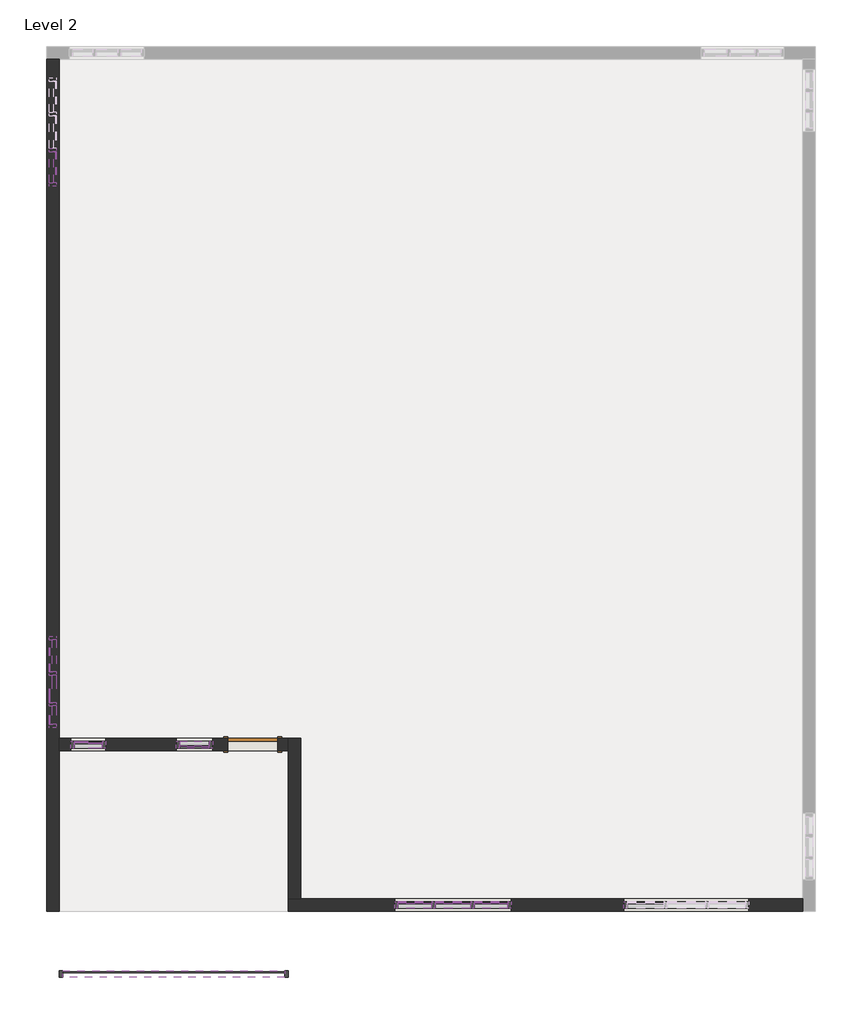
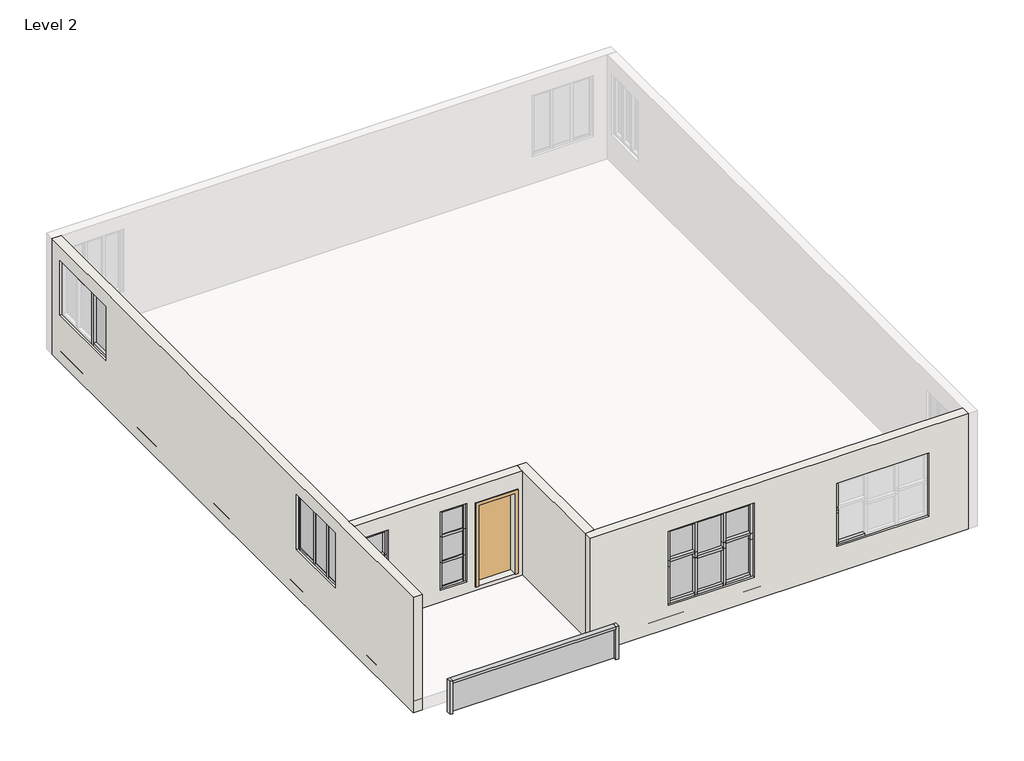
# One storey, part 1 of 2: 64 members, 17 plates, 4 walls, 1 door.
"""IFC4 building model written with IfcOpenShell, lengths in millimetres."""

from ifc_helpers import new_model, si_unit, frame, origin, place, context, project, spatial, polyline, outline, extrude, faceted_brep, transform, mapped, element, save
from components import door_0ca8825f, member_2ebf4a73, member_c33c434a, member_7fd687a9, member_90750a43, member_e53b78c9, member_5215b92c, member_3f0e0172, member_f6f0dfdd, member_f8dc38bf, member_876f8f00, member_a400357f, member_6f432376, member_04a79ac1, member_b1615173, member_02b8d6b6, member_e5d39754, member_6045db05, member_ce41b455, member_0c7d0587, member_4df5bd8f, member_19666b72, member_6e6cbf30, member_3d7cb871, member_3cc62806, member_2ad165f7, member_377cf5f8, member_b281fab0, member_bdfbb35d, member_c769c9ba, member_bec57569, member_6f9d7b88, system_panel_glazed_a7448bf8, system_panel_glazed_e40eab22, system_panel_glazed_7c0c5eec, system_panel_glazed_eaaab531, system_panel_glazed_8162a39b, system_panel_glazed_8a587fcc, system_panel_glazed_8182dcf9, system_panel_glazed_b409b60d, system_panel_glazed_f2280d1b, system_panel_glazed_618baec5, system_panel_glazed_209ba7b6, system_panel_glazed_68ae91f2, system_panel_glazed_7aae5990

model = new_model("IFC4")

# Units and contexts
model_context = context("Model", 3, world=origin())
ifc_project = project(units=[si_unit("LENGTHUNIT", "METRE", prefix="MILLI")], contexts=[model_context])

# Site, building, storey
site = spatial("IfcSite", under=ifc_project)
building = spatial("IfcBuilding", under=site)
storey = spatial("IfcBuildingStorey", under=building, Name="Level 2", Elevation=3048.0)

# Door
placement = place(None, origin())
door_shape = door_0ca8825f(model_context)
element("IfcDoor", 1, ObjectType="Single-Flush : 36\" x 84\"", at=placement, inside=storey, context=model_context, shape_type="MappedRepresentation", body=[
    mapped(door_shape, transform((-18079.9097681, -11198.7339922, 3454.4), x_axis=(1.0, 0.0, 0.0), y_axis=(0.0, 1.0, 0.0), z_axis=(0.0, 0.0, 1.0))),
])

# Members
member_shape = member_2ebf4a73(model_context)
element("IfcMember", 2, ObjectType="Rectangular Mullion : 2.5\" x 5\" rectangular", at=placement, inside=storey, context=model_context, shape_type="MappedRepresentation", body=[
    mapped(member_shape, transform((-21737.5097681, -9935.0839922, 5757.8760039), x_axis=(0.0, 0.0, 1.0), y_axis=(1.0, 0.0, 0.0), z_axis=(0.0, 1.0, 0.0))),
])
element("IfcMember", 3, ObjectType="Rectangular Mullion : 2.5\" x 5\" rectangular", at=placement, inside=storey, context=model_context, shape_type="MappedRepresentation", body=[
    mapped(member_shape, transform((-21737.5097681, -10430.3839922, 4301.2247959), x_axis=(0.0, 0.0, -1.0), y_axis=(1.0, 0.0, 0.0), z_axis=(0.0, -1.0, 0.0))),
])
member_2_shape = member_c33c434a(model_context)
element("IfcMember", 4, ObjectType="Rectangular Mullion : 2.5\" x 5\" rectangular", at=placement, inside=storey, context=model_context, shape_type="MappedRepresentation", body=[
    mapped(member_2_shape, transform((-11234.6097681, -14132.4339922, 3732.481147), x_axis=(0.0, 0.0, -1.0), y_axis=(0.0, -1.0, 0.0), z_axis=(-1.0, 0.0, 0.0))),
])
member_3_shape = member_7fd687a9(model_context)
element("IfcMember", 5, ObjectType="Rectangular Mullion : 2.5\" x 5\" rectangular", at=placement, inside=storey, context=model_context, shape_type="MappedRepresentation", body=[
    mapped(member_3_shape, transform((-20835.8097681, -11198.7339922, 5713.3390555), x_axis=(0.0, 0.0, 1.0), y_axis=(0.0, -1.0, 0.0), z_axis=(1.0, 0.0, 0.0))),
])
member_4_shape = member_90750a43(model_context)
element("IfcMember", 6, ObjectType="Rectangular Mullion : 2.5\" x 5\" rectangular", at=placement, inside=storey, context=model_context, shape_type="MappedRepresentation", body=[
    mapped(member_4_shape, transform((-20835.8097681, -11198.7339922, 5044.6242619), x_axis=(0.0, 0.0, 1.0), y_axis=(0.0, -1.0, 0.0), z_axis=(1.0, 0.0, 0.0))),
])
element("IfcMember", 7, ObjectType="Rectangular Mullion : 2.5\" x 5\" rectangular", at=placement, inside=storey, context=model_context, shape_type="MappedRepresentation", body=[
    mapped(member_4_shape, transform((-20835.8097681, -11198.7339922, 4375.9094684), x_axis=(0.0, 0.0, 1.0), y_axis=(0.0, -1.0, 0.0), z_axis=(1.0, 0.0, 0.0))),
])
element("IfcMember", 8, ObjectType="Rectangular Mullion : 2.5\" x 5\" rectangular", at=placement, inside=storey, context=model_context, shape_type="MappedRepresentation", body=[
    mapped(member_3_shape, transform((-21343.8097681, -11198.7339922, 3707.1946748), x_axis=(0.0, 0.0, -1.0), y_axis=(0.0, -1.0, 0.0), z_axis=(-1.0, 0.0, 0.0))),
])
member_5_shape = member_e53b78c9(model_context)
element("IfcMember", 9, ObjectType="Rectangular Mullion : 2.5\" x 5\" rectangular", at=placement, inside=storey, context=model_context, shape_type="MappedRepresentation", body=[
    mapped(member_5_shape, transform((-14098.4597681, -14132.4339922, 4627.6072298), x_axis=(0.0, 0.0, 1.0), y_axis=(0.0, -1.0, 0.0), z_axis=(1.0, 0.0, 0.0))),
])
member_6_shape = member_5215b92c(model_context)
element("IfcMember", 10, ObjectType="Rectangular Mullion : 2.5\" x 5\" rectangular", at=placement, inside=storey, context=model_context, shape_type="MappedRepresentation", body=[
    mapped(member_6_shape, transform((-14098.4597681, -14132.4339922, 5607.3382011), x_axis=(0.0, 0.0, 1.0), y_axis=(0.0, -1.0, 0.0), z_axis=(1.0, 0.0, 0.0))),
])
member_7_shape = member_3f0e0172(model_context)
element("IfcMember", 11, ObjectType="Rectangular Mullion : 2.5\" x 5\" rectangular", at=placement, inside=storey, context=model_context, shape_type="MappedRepresentation", body=[
    mapped(member_7_shape, transform((-14809.6597681, -14132.4339922, 5607.3382011), x_axis=(0.0, 0.0, 1.0), y_axis=(0.0, -1.0, 0.0), z_axis=(1.0, 0.0, 0.0))),
])
element("IfcMember", 12, ObjectType="Rectangular Mullion : 2.5\" x 5\" rectangular", at=placement, inside=storey, context=model_context, shape_type="MappedRepresentation", body=[
    mapped(member_7_shape, transform((-13419.0097681, -14132.4339922, 5607.3382011), x_axis=(0.0, 0.0, 1.0), y_axis=(0.0, -1.0, 0.0), z_axis=(1.0, 0.0, 0.0))),
])
member_8_shape = member_f6f0dfdd(model_context)
element("IfcMember", 13, ObjectType="Rectangular Mullion : 2.5\" x 5\" rectangular", at=placement, inside=storey, context=model_context, shape_type="MappedRepresentation", body=[
    mapped(member_8_shape, transform((-14777.9097681, -14132.4339922, 4627.6072298), x_axis=(1.0, 0.0, 0.0), y_axis=(0.0, -1.0, 0.0), z_axis=(0.0, 0.0, -1.0))),
])
element("IfcMember", 14, ObjectType="Rectangular Mullion : 2.5\" x 5\" rectangular", at=placement, inside=storey, context=model_context, shape_type="MappedRepresentation", body=[
    mapped(member_8_shape, transform((-14066.7097681, -14132.4339922, 4627.6072298), x_axis=(1.0, 0.0, 0.0), y_axis=(0.0, -1.0, 0.0), z_axis=(0.0, 0.0, -1.0))),
])
member_9_shape = member_f8dc38bf(model_context)
element("IfcMember", 15, ObjectType="Rectangular Mullion : 2.5\" x 5\" rectangular", at=placement, inside=storey, context=model_context, shape_type="MappedRepresentation", body=[
    mapped(member_9_shape, transform((-13419.0097681, -14132.4339922, 4780.0072298), x_axis=(0.0, 0.0, 1.0), y_axis=(0.0, -1.0, 0.0), z_axis=(1.0, 0.0, 0.0))),
])
element("IfcMember", 16, ObjectType="Rectangular Mullion : 2.5\" x 5\" rectangular", at=placement, inside=storey, context=model_context, shape_type="MappedRepresentation", body=[
    mapped(member_9_shape, transform((-14809.6597681, -14132.4339922, 4780.0072298), x_axis=(0.0, 0.0, 1.0), y_axis=(0.0, -1.0, 0.0), z_axis=(1.0, 0.0, 0.0))),
])
member_10_shape = member_876f8f00(model_context)
element("IfcMember", 17, ObjectType="Rectangular Mullion : 2.5\" x 5\" rectangular", at=placement, inside=storey, context=model_context, shape_type="MappedRepresentation", body=[
    mapped(member_10_shape, transform((-13355.5097681, -14132.4339922, 4627.6072298), x_axis=(1.0, 0.0, 0.0), y_axis=(0.0, -1.0, 0.0), z_axis=(0.0, 0.0, -1.0))),
])
element("IfcMember", 18, ObjectType="Rectangular Mullion : 2.5\" x 5\" rectangular", at=placement, inside=storey, context=model_context, shape_type="MappedRepresentation", body=[
    mapped(member_10_shape, transform((-15489.1097681, -14132.4339922, 4780.0072298), x_axis=(-1.0, 0.0, 0.0), y_axis=(0.0, -1.0, 0.0), z_axis=(0.0, 0.0, 1.0))),
])
element("IfcMember", 19, ObjectType="Rectangular Mullion : 2.5\" x 5\" rectangular", at=placement, inside=storey, context=model_context, shape_type="MappedRepresentation", body=[
    mapped(member_7_shape, transform((-14034.9597681, -14132.4339922, 3647.8762585), x_axis=(0.0, 0.0, -1.0), y_axis=(0.0, -1.0, 0.0), z_axis=(-1.0, 0.0, 0.0))),
])
element("IfcMember", 20, ObjectType="Rectangular Mullion : 2.5\" x 5\" rectangular", at=placement, inside=storey, context=model_context, shape_type="MappedRepresentation", body=[
    mapped(member_7_shape, transform((-15425.6097681, -14132.4339922, 3647.8762585), x_axis=(0.0, 0.0, -1.0), y_axis=(0.0, -1.0, 0.0), z_axis=(-1.0, 0.0, 0.0))),
])
element("IfcMember", 21, ObjectType="Rectangular Mullion : 2.5\" x 5\" rectangular", at=placement, inside=storey, context=model_context, shape_type="MappedRepresentation", body=[
    mapped(member_6_shape, transform((-14746.1597681, -14132.4339922, 3647.8762585), x_axis=(0.0, 0.0, -1.0), y_axis=(0.0, -1.0, 0.0), z_axis=(-1.0, 0.0, 0.0))),
])
member_11_shape = member_a400357f(model_context)
element("IfcMember", 22, ObjectType="Rectangular Mullion : 2.5\" x 5\" rectangular", at=placement, inside=storey, context=model_context, shape_type="MappedRepresentation", body=[
    mapped(member_11_shape, transform((-21737.5097681, -295.7839922, 5718.9037492), x_axis=(0.0, 0.0, 1.0), y_axis=(-1.0, 0.0, 0.0), z_axis=(0.0, -1.0, 0.0))),
])
member_12_shape = member_6f432376(model_context)
element("IfcMember", 23, ObjectType="Rectangular Mullion : 2.5\" x 5\" rectangular", at=placement, inside=storey, context=model_context, shape_type="MappedRepresentation", body=[
    mapped(member_12_shape, transform((-21737.5097681, -924.4339922, 5718.9037492), x_axis=(0.0, 0.0, 1.0), y_axis=(-1.0, 0.0, 0.0), z_axis=(0.0, -1.0, 0.0))),
])
member_13_shape = member_04a79ac1(model_context)
element("IfcMember", 24, ObjectType="Rectangular Mullion : 2.5\" x 5\" rectangular", at=placement, inside=storey, context=model_context, shape_type="MappedRepresentation", body=[
    mapped(member_13_shape, transform((-21737.5097681, -327.5339922, 4287.8866443), x_axis=(0.0, -1.0, 0.0), y_axis=(-1.0, 0.0, 0.0), z_axis=(0.0, 0.0, -1.0))),
])
element("IfcMember", 25, ObjectType="Rectangular Mullion : 2.5\" x 5\" rectangular", at=placement, inside=storey, context=model_context, shape_type="MappedRepresentation", body=[
    mapped(member_12_shape, transform((-21737.5097681, -359.2839922, 4287.8866443), x_axis=(0.0, 0.0, -1.0), y_axis=(-1.0, 0.0, 0.0), z_axis=(0.0, 1.0, 0.0))),
])
member_14_shape = member_b1615173(model_context)
element("IfcMember", 26, ObjectType="Rectangular Mullion : 2.5\" x 5\" rectangular", at=placement, inside=storey, context=model_context, shape_type="MappedRepresentation", body=[
    mapped(member_14_shape, transform((-21737.5097681, -987.9339922, 4287.8866443), x_axis=(0.0, -1.0, 0.0), y_axis=(-1.0, 0.0, 0.0), z_axis=(0.0, 0.0, -1.0))),
])
member_15_shape = member_02b8d6b6(model_context)
element("IfcMember", 27, ObjectType="Rectangular Mullion : 2.5\" x 5\" rectangular", at=placement, inside=storey, context=model_context, shape_type="MappedRepresentation", body=[
    mapped(member_15_shape, transform((-21737.5097681, -10493.8839922, 5757.8760039), x_axis=(0.0, 0.0, 1.0), y_axis=(1.0, 0.0, 0.0), z_axis=(0.0, 1.0, 0.0))),
])
member_16_shape = member_e5d39754(model_context)
element("IfcMember", 28, ObjectType="Rectangular Mullion : 2.5\" x 5\" rectangular", at=placement, inside=storey, context=model_context, shape_type="MappedRepresentation", body=[
    mapped(member_16_shape, transform((-21737.5097681, -9281.0339922, 5757.8760039), x_axis=(0.0, 0.0, 1.0), y_axis=(1.0, 0.0, 0.0), z_axis=(0.0, 1.0, 0.0))),
])
member_17_shape = member_6045db05(model_context)
element("IfcMember", 29, ObjectType="Rectangular Mullion : 2.5\" x 5\" rectangular", at=placement, inside=storey, context=model_context, shape_type="MappedRepresentation", body=[
    mapped(member_17_shape, transform((-21737.5097681, -9903.3339922, 4301.2247959), x_axis=(0.0, 1.0, 0.0), y_axis=(1.0, 0.0, 0.0), z_axis=(0.0, 0.0, -1.0))),
])
element("IfcMember", 30, ObjectType="Rectangular Mullion : 2.5\" x 5\" rectangular", at=placement, inside=storey, context=model_context, shape_type="MappedRepresentation", body=[
    mapped(member_17_shape, transform((-21737.5097681, -10462.1339922, 4301.2247959), x_axis=(0.0, 1.0, 0.0), y_axis=(1.0, 0.0, 0.0), z_axis=(0.0, 0.0, -1.0))),
])
element("IfcMember", 31, ObjectType="Rectangular Mullion : 2.5\" x 5\" rectangular", at=placement, inside=storey, context=model_context, shape_type="MappedRepresentation", body=[
    mapped(member_16_shape, transform((-21737.5097681, -9871.5839922, 4301.2247959), x_axis=(0.0, 0.0, -1.0), y_axis=(1.0, 0.0, 0.0), z_axis=(0.0, -1.0, 0.0))),
])
element("IfcMember", 32, ObjectType="Rectangular Mullion : 2.5\" x 5\" rectangular", at=placement, inside=storey, context=model_context, shape_type="MappedRepresentation", body=[
    mapped(member_15_shape, transform((-21737.5097681, -10830.4339922, 4301.2247959), x_axis=(0.0, 0.0, -1.0), y_axis=(1.0, 0.0, 0.0), z_axis=(0.0, -1.0, 0.0))),
])
member_18_shape = member_ce41b455(model_context)
element("IfcMember", 33, ObjectType="Rectangular Mullion : 2.5\" x 5\" rectangular", at=placement, inside=storey, context=model_context, shape_type="MappedRepresentation", body=[
    mapped(member_18_shape, transform((-21737.5097681, -10893.9339922, 5757.8760039), x_axis=(0.0, -1.0, 0.0), y_axis=(1.0, 0.0, 0.0), z_axis=(0.0, 0.0, 1.0))),
])
element("IfcMember", 34, ObjectType="Rectangular Mullion : 2.5\" x 5\" rectangular", at=placement, inside=storey, context=model_context, shape_type="MappedRepresentation", body=[
    mapped(member_18_shape, transform((-21737.5097681, -9217.5339922, 4301.2247959), x_axis=(0.0, 1.0, 0.0), y_axis=(1.0, 0.0, 0.0), z_axis=(0.0, 0.0, -1.0))),
])
member_19_shape = member_0c7d0587(model_context)
element("IfcMember", 35, ObjectType="Rectangular Mullion : 2.5\" x 5\" rectangular", at=placement, inside=storey, context=model_context, shape_type="MappedRepresentation", body=[
    mapped(member_19_shape, transform((-14777.9097681, -14132.4339922, 4780.0072298), x_axis=(1.0, 0.0, 0.0), y_axis=(0.0, -1.0, 0.0), z_axis=(0.0, 0.0, -1.0))),
])
element("IfcMember", 36, ObjectType="Rectangular Mullion : 2.5\" x 5\" rectangular", at=placement, inside=storey, context=model_context, shape_type="MappedRepresentation", body=[
    mapped(member_19_shape, transform((-14066.7097681, -14132.4339922, 4780.0072298), x_axis=(1.0, 0.0, 0.0), y_axis=(0.0, -1.0, 0.0), z_axis=(0.0, 0.0, -1.0))),
])
member_20_shape = member_4df5bd8f(model_context)
element("IfcMember", 37, ObjectType="Rectangular Mullion : 2.5\" x 5\" rectangular", at=placement, inside=storey, context=model_context, shape_type="MappedRepresentation", body=[
    mapped(member_20_shape, transform((-15489.1097681, -14132.4339922, 5607.3382011), x_axis=(-1.0, 0.0, 0.0), y_axis=(0.0, -1.0, 0.0), z_axis=(0.0, 0.0, 1.0))),
])
element("IfcMember", 38, ObjectType="Rectangular Mullion : 2.5\" x 5\" rectangular", at=placement, inside=storey, context=model_context, shape_type="MappedRepresentation", body=[
    mapped(member_20_shape, transform((-13355.5097681, -14132.4339922, 4780.0072298), x_axis=(1.0, 0.0, 0.0), y_axis=(0.0, -1.0, 0.0), z_axis=(0.0, 0.0, -1.0))),
])
member_21_shape = member_19666b72(model_context)
element("IfcMember", 39, ObjectType="Rectangular Mullion : 2.5\" x 5\" rectangular", at=placement, inside=storey, context=model_context, shape_type="MappedRepresentation", body=[
    mapped(member_21_shape, transform((-14777.9097681, -14132.4339922, 3647.8762585), x_axis=(1.0, 0.0, 0.0), y_axis=(0.0, -1.0, 0.0), z_axis=(0.0, 0.0, -1.0))),
])
element("IfcMember", 40, ObjectType="Rectangular Mullion : 2.5\" x 5\" rectangular", at=placement, inside=storey, context=model_context, shape_type="MappedRepresentation", body=[
    mapped(member_21_shape, transform((-14066.7097681, -14132.4339922, 3647.8762585), x_axis=(1.0, 0.0, 0.0), y_axis=(0.0, -1.0, 0.0), z_axis=(0.0, 0.0, -1.0))),
])
member_22_shape = member_6e6cbf30(model_context)
element("IfcMember", 41, ObjectType="Rectangular Mullion : 2.5\" x 5\" rectangular", at=placement, inside=storey, context=model_context, shape_type="MappedRepresentation", body=[
    mapped(member_22_shape, transform((-15489.1097681, -14132.4339922, 4627.6072298), x_axis=(-1.0, 0.0, 0.0), y_axis=(0.0, -1.0, 0.0), z_axis=(0.0, 0.0, 1.0))),
])
element("IfcMember", 42, ObjectType="Rectangular Mullion : 2.5\" x 5\" rectangular", at=placement, inside=storey, context=model_context, shape_type="MappedRepresentation", body=[
    mapped(member_22_shape, transform((-13355.5097681, -14132.4339922, 3647.8762585), x_axis=(1.0, 0.0, 0.0), y_axis=(0.0, -1.0, 0.0), z_axis=(0.0, 0.0, -1.0))),
])
member_23_shape = member_3d7cb871(model_context)
element("IfcMember", 43, ObjectType="Rectangular Mullion : 2.5\" x 5\" rectangular", at=placement, inside=storey, context=model_context, shape_type="MappedRepresentation", body=[
    mapped(member_23_shape, transform((-11298.1097681, -14132.4339922, 4641.1200239), x_axis=(-1.0, 0.0, 0.0), y_axis=(0.0, -1.0, 0.0), z_axis=(0.0, 0.0, 1.0))),
])
element("IfcMember", 44, ObjectType="Rectangular Mullion : 2.5\" x 5\" rectangular", at=placement, inside=storey, context=model_context, shape_type="MappedRepresentation", body=[
    mapped(member_23_shape, transform((-11298.1097681, -14132.4339922, 4717.3200239), x_axis=(-1.0, 0.0, 0.0), y_axis=(0.0, -1.0, 0.0), z_axis=(0.0, 0.0, 1.0))),
])
member_24_shape = member_3cc62806(model_context)
element("IfcMember", 45, ObjectType="Rectangular Mullion : 2.5\" x 5\" rectangular", at=placement, inside=storey, context=model_context, shape_type="MappedRepresentation", body=[
    mapped(member_24_shape, transform((-11298.1097681, -14132.4339922, 5397.3589008), x_axis=(-1.0, 0.0, 0.0), y_axis=(0.0, -1.0, 0.0), z_axis=(0.0, 0.0, 1.0))),
])
member_25_shape = member_2ad165f7(model_context)
element("IfcMember", 46, ObjectType="Rectangular Mullion : 2.5\" x 5\" rectangular", at=placement, inside=storey, context=model_context, shape_type="MappedRepresentation", body=[
    mapped(member_25_shape, transform((-11298.1097681, -14132.4339922, 4564.9200239), x_axis=(-1.0, 0.0, 0.0), y_axis=(0.0, -1.0, 0.0), z_axis=(0.0, 0.0, 1.0))),
])
member_26_shape = member_377cf5f8(model_context)
element("IfcMember", 47, ObjectType="Rectangular Mullion : 2.5\" x 5\" rectangular", at=placement, inside=storey, context=model_context, shape_type="MappedRepresentation", body=[
    mapped(member_26_shape, transform((-20772.3097681, -11198.7339922, 5044.6242619), x_axis=(1.0, 0.0, 0.0), y_axis=(0.0, -1.0, 0.0), z_axis=(0.0, 0.0, -1.0))),
])
element("IfcMember", 48, ObjectType="Rectangular Mullion : 2.5\" x 5\" rectangular", at=placement, inside=storey, context=model_context, shape_type="MappedRepresentation", body=[
    mapped(member_26_shape, transform((-21407.3097681, -11198.7339922, 5713.3390555), x_axis=(-1.0, 0.0, 0.0), y_axis=(0.0, -1.0, 0.0), z_axis=(0.0, 0.0, 1.0))),
])
element("IfcMember", 49, ObjectType="Rectangular Mullion : 2.5\" x 5\" rectangular", at=placement, inside=storey, context=model_context, shape_type="MappedRepresentation", body=[
    mapped(member_26_shape, transform((-20772.3097681, -11198.7339922, 4375.9094684), x_axis=(1.0, 0.0, 0.0), y_axis=(0.0, -1.0, 0.0), z_axis=(0.0, 0.0, -1.0))),
])
element("IfcMember", 50, ObjectType="Rectangular Mullion : 2.5\" x 5\" rectangular", at=placement, inside=storey, context=model_context, shape_type="MappedRepresentation", body=[
    mapped(member_26_shape, transform((-21407.3097681, -11198.7339922, 5044.6242619), x_axis=(-1.0, 0.0, 0.0), y_axis=(0.0, -1.0, 0.0), z_axis=(0.0, 0.0, 1.0))),
])
element("IfcMember", 51, ObjectType="Rectangular Mullion : 2.5\" x 5\" rectangular", at=placement, inside=storey, context=model_context, shape_type="MappedRepresentation", body=[
    mapped(member_26_shape, transform((-20772.3097681, -11198.7339922, 3707.1946748), x_axis=(1.0, 0.0, 0.0), y_axis=(0.0, -1.0, 0.0), z_axis=(0.0, 0.0, -1.0))),
])
element("IfcMember", 52, ObjectType="Rectangular Mullion : 2.5\" x 5\" rectangular", at=placement, inside=storey, context=model_context, shape_type="MappedRepresentation", body=[
    mapped(member_26_shape, transform((-21407.3097681, -11198.7339922, 4375.9094684), x_axis=(-1.0, 0.0, 0.0), y_axis=(0.0, -1.0, 0.0), z_axis=(0.0, 0.0, 1.0))),
])
member_27_shape = member_b281fab0(model_context)
element("IfcMember", 53, ObjectType="Rectangular Mullion : 2.5\" x 5\" rectangular", at=placement, inside=storey, context=model_context, shape_type="MappedRepresentation", body=[
    mapped(member_27_shape, transform((-19413.4097681, -11198.7339922, 5730.4529017), x_axis=(0.0, 0.0, 1.0), y_axis=(0.0, 1.0, 0.0), z_axis=(-1.0, 0.0, 0.0))),
])
member_28_shape = member_bdfbb35d(model_context)
element("IfcMember", 54, ObjectType="Rectangular Mullion : 2.5\" x 5\" rectangular", at=placement, inside=storey, context=model_context, shape_type="MappedRepresentation", body=[
    mapped(member_28_shape, transform((-19413.4097681, -11198.7339922, 5039.9788679), x_axis=(0.0, 0.0, 1.0), y_axis=(0.0, 1.0, 0.0), z_axis=(-1.0, 0.0, 0.0))),
])
element("IfcMember", 55, ObjectType="Rectangular Mullion : 2.5\" x 5\" rectangular", at=placement, inside=storey, context=model_context, shape_type="MappedRepresentation", body=[
    mapped(member_28_shape, transform((-19413.4097681, -11198.7339922, 4349.5048342), x_axis=(0.0, 0.0, 1.0), y_axis=(0.0, 1.0, 0.0), z_axis=(-1.0, 0.0, 0.0))),
])
member_29_shape = member_c769c9ba(model_context)
element("IfcMember", 56, ObjectType="Rectangular Mullion : 2.5\" x 5\" rectangular", at=placement, inside=storey, context=model_context, shape_type="MappedRepresentation", body=[
    mapped(member_29_shape, transform((-18816.5097681, -11198.7339922, 5730.4529017), x_axis=(1.0, 0.0, 0.0), y_axis=(0.0, 1.0, 0.0), z_axis=(0.0, 0.0, 1.0))),
])
element("IfcMember", 57, ObjectType="Rectangular Mullion : 2.5\" x 5\" rectangular", at=placement, inside=storey, context=model_context, shape_type="MappedRepresentation", body=[
    mapped(member_29_shape, transform((-19476.9097681, -11198.7339922, 5039.9788679), x_axis=(-1.0, 0.0, 0.0), y_axis=(0.0, 1.0, 0.0), z_axis=(0.0, 0.0, -1.0))),
])
element("IfcMember", 58, ObjectType="Rectangular Mullion : 2.5\" x 5\" rectangular", at=placement, inside=storey, context=model_context, shape_type="MappedRepresentation", body=[
    mapped(member_29_shape, transform((-18816.5097681, -11198.7339922, 5039.9788679), x_axis=(1.0, 0.0, 0.0), y_axis=(0.0, 1.0, 0.0), z_axis=(0.0, 0.0, 1.0))),
])
element("IfcMember", 59, ObjectType="Rectangular Mullion : 2.5\" x 5\" rectangular", at=placement, inside=storey, context=model_context, shape_type="MappedRepresentation", body=[
    mapped(member_29_shape, transform((-19476.9097681, -11198.7339922, 4349.5048342), x_axis=(-1.0, 0.0, 0.0), y_axis=(0.0, 1.0, 0.0), z_axis=(0.0, 0.0, -1.0))),
])
element("IfcMember", 60, ObjectType="Rectangular Mullion : 2.5\" x 5\" rectangular", at=placement, inside=storey, context=model_context, shape_type="MappedRepresentation", body=[
    mapped(member_27_shape, transform((-18880.0097681, -11198.7339922, 3659.0308004), x_axis=(0.0, 0.0, -1.0), y_axis=(0.0, 1.0, 0.0), z_axis=(1.0, 0.0, 0.0))),
])
element("IfcMember", 61, ObjectType="Rectangular Mullion : 2.5\" x 5\" rectangular", at=placement, inside=storey, context=model_context, shape_type="MappedRepresentation", body=[
    mapped(member_29_shape, transform((-18816.5097681, -11198.7339922, 4349.5048342), x_axis=(1.0, 0.0, 0.0), y_axis=(0.0, 1.0, 0.0), z_axis=(0.0, 0.0, 1.0))),
])
element("IfcMember", 62, ObjectType="Rectangular Mullion : 2.5\" x 5\" rectangular", at=placement, inside=storey, context=model_context, shape_type="MappedRepresentation", body=[
    mapped(member_29_shape, transform((-19476.9097681, -11198.7339922, 3659.0308004), x_axis=(-1.0, 0.0, 0.0), y_axis=(0.0, 1.0, 0.0), z_axis=(0.0, 0.0, -1.0))),
])
member_30_shape = member_bec57569(model_context)
element("IfcMember", 63, ObjectType="Rectangular Mullion : 2.5\" x 5\" rectangular", at=placement, inside=storey, context=model_context, shape_type="MappedRepresentation", body=[
    mapped(member_30_shape, transform((-17432.2097681, -15394.0454888, 3659.0308004), x_axis=(1.0, 0.0, 0.0), y_axis=(0.0, -1.0, 0.0), z_axis=(0.0, 0.0, -1.0))),
])
member_31_shape = member_6f9d7b88(model_context)
element("IfcMember", 64, ObjectType="Rectangular Mullion : 2.5\" x 5\" rectangular", at=placement, inside=storey, context=model_context, shape_type="MappedRepresentation", body=[
    mapped(member_31_shape, transform((-17495.7097681, -15394.0454888, 4526.6965957), x_axis=(0.0, 0.0, 1.0), y_axis=(0.0, -1.0, 0.0), z_axis=(1.0, 0.0, 0.0))),
])
element("IfcMember", 65, ObjectType="Rectangular Mullion : 2.5\" x 5\" rectangular", at=placement, inside=storey, context=model_context, shape_type="MappedRepresentation", body=[
    mapped(member_30_shape, transform((-21623.2097681, -15394.0454888, 4526.6965957), x_axis=(-1.0, 0.0, 0.0), y_axis=(0.0, -1.0, 0.0), z_axis=(0.0, 0.0, 1.0))),
])

# Plates
system_panel_glazed_shape = system_panel_glazed_a7448bf8(model_context)
element("IfcPlate", 66, ObjectType="System Panel : Glazed", at=placement, inside=storey, context=model_context, shape_type="MappedRepresentation", body=[
    mapped(system_panel_glazed_shape, transform((-21737.5097681, -641.8589922, 4351.3866443), x_axis=(0.0, -1.0, 0.0), y_axis=(1.0, 0.0, 0.0), z_axis=(0.0, 0.0, 1.0))),
])
system_panel_glazed_2_shape = system_panel_glazed_e40eab22(model_context)
element("IfcPlate", 67, ObjectType="System Panel : Glazed", at=placement, inside=storey, context=model_context, shape_type="MappedRepresentation", body=[
    mapped(system_panel_glazed_2_shape, transform((-21737.5097681, -10662.1589922, 4364.7247959), x_axis=(0.0, 1.0, 0.0), y_axis=(-1.0, 0.0, 0.0), z_axis=(0.0, 0.0, 1.0))),
])
system_panel_glazed_3_shape = system_panel_glazed_7c0c5eec(model_context)
element("IfcPlate", 68, ObjectType="System Panel : Glazed", at=placement, inside=storey, context=model_context, shape_type="MappedRepresentation", body=[
    mapped(system_panel_glazed_3_shape, transform((-21737.5097681, -9576.3089922, 4364.7247959), x_axis=(0.0, 1.0, 0.0), y_axis=(-1.0, 0.0, 0.0), z_axis=(0.0, 0.0, 1.0))),
])
system_panel_glazed_4_shape = system_panel_glazed_eaaab531(model_context)
element("IfcPlate", 69, ObjectType="System Panel : Glazed", at=placement, inside=storey, context=model_context, shape_type="MappedRepresentation", body=[
    mapped(system_panel_glazed_4_shape, transform((-21737.5097681, -10182.7339922, 4364.7247959), x_axis=(0.0, 1.0, 0.0), y_axis=(-1.0, 0.0, 0.0), z_axis=(0.0, 0.0, 1.0))),
])
system_panel_glazed_5_shape = system_panel_glazed_8162a39b(model_context)
element("IfcPlate", 70, ObjectType="System Panel : Glazed", at=placement, inside=storey, context=model_context, shape_type="MappedRepresentation", body=[
    mapped(system_panel_glazed_5_shape, transform((-14422.3097681, -14132.4339922, 4659.3572298), x_axis=(1.0, 0.0, 0.0), y_axis=(0.0, 1.0, 0.0), z_axis=(0.0, 0.0, 1.0))),
])
system_panel_glazed_6_shape = system_panel_glazed_8a587fcc(model_context)
element("IfcPlate", 71, ObjectType="System Panel : Glazed", at=placement, inside=storey, context=model_context, shape_type="MappedRepresentation", body=[
    mapped(system_panel_glazed_6_shape, transform((-15117.6347681, -14132.4339922, 4811.7572298), x_axis=(1.0, 0.0, 0.0), y_axis=(0.0, 1.0, 0.0), z_axis=(0.0, 0.0, 1.0))),
])
element("IfcPlate", 72, ObjectType="System Panel : Glazed", at=placement, inside=storey, context=model_context, shape_type="MappedRepresentation", body=[
    mapped(system_panel_glazed_6_shape, transform((-13726.9847681, -14132.4339922, 4811.7572298), x_axis=(1.0, 0.0, 0.0), y_axis=(0.0, 1.0, 0.0), z_axis=(0.0, 0.0, 1.0))),
])
system_panel_glazed_7_shape = system_panel_glazed_8182dcf9(model_context)
element("IfcPlate", 73, ObjectType="System Panel : Glazed", at=placement, inside=storey, context=model_context, shape_type="MappedRepresentation", body=[
    mapped(system_panel_glazed_7_shape, transform((-15117.6347681, -14132.4339922, 3711.3762585), x_axis=(1.0, 0.0, 0.0), y_axis=(0.0, 1.0, 0.0), z_axis=(0.0, 0.0, 1.0))),
])
element("IfcPlate", 74, ObjectType="System Panel : Glazed", at=placement, inside=storey, context=model_context, shape_type="MappedRepresentation", body=[
    mapped(system_panel_glazed_7_shape, transform((-13726.9847681, -14132.4339922, 3711.3762585), x_axis=(1.0, 0.0, 0.0), y_axis=(0.0, 1.0, 0.0), z_axis=(0.0, 0.0, 1.0))),
])
system_panel_glazed_8_shape = system_panel_glazed_b409b60d(model_context)
element("IfcPlate", 75, ObjectType="System Panel : Glazed", at=placement, inside=storey, context=model_context, shape_type="MappedRepresentation", body=[
    mapped(system_panel_glazed_8_shape, transform((-14422.3097681, -14132.4339922, 3711.3762585), x_axis=(1.0, 0.0, 0.0), y_axis=(0.0, 1.0, 0.0), z_axis=(0.0, 0.0, 1.0))),
])
system_panel_glazed_9_shape = system_panel_glazed_f2280d1b(model_context)
element("IfcPlate", 76, ObjectType="System Panel : Glazed", at=placement, inside=storey, context=model_context, shape_type="MappedRepresentation", body=[
    mapped(system_panel_glazed_9_shape, transform((-21089.8097681, -11198.7339922, 3770.6946748), x_axis=(1.0, 0.0, 0.0), y_axis=(0.0, 1.0, 0.0), z_axis=(0.0, 0.0, 1.0))),
])
element("IfcPlate", 77, ObjectType="System Panel : Glazed", at=placement, inside=storey, context=model_context, shape_type="MappedRepresentation", body=[
    mapped(system_panel_glazed_9_shape, transform((-21089.8097681, -11198.7339922, 5076.3742619), x_axis=(1.0, 0.0, 0.0), y_axis=(0.0, 1.0, 0.0), z_axis=(0.0, 0.0, 1.0))),
])
system_panel_glazed_10_shape = system_panel_glazed_618baec5(model_context)
element("IfcPlate", 78, ObjectType="System Panel : Glazed", at=placement, inside=storey, context=model_context, shape_type="MappedRepresentation", body=[
    mapped(system_panel_glazed_10_shape, transform((-21089.8097681, -11198.7339922, 4407.6594684), x_axis=(1.0, 0.0, 0.0), y_axis=(0.0, 1.0, 0.0), z_axis=(0.0, 0.0, 1.0))),
])
system_panel_glazed_11_shape = system_panel_glazed_209ba7b6(model_context)
element("IfcPlate", 79, ObjectType="System Panel : Glazed", at=placement, inside=storey, context=model_context, shape_type="MappedRepresentation", body=[
    mapped(system_panel_glazed_11_shape, transform((-19146.7097681, -11198.7339922, 3722.5308004), x_axis=(-1.0, 0.0, 0.0), y_axis=(0.0, -1.0, 0.0), z_axis=(0.0, 0.0, 1.0))),
])
element("IfcPlate", 80, ObjectType="System Panel : Glazed", at=placement, inside=storey, context=model_context, shape_type="MappedRepresentation", body=[
    mapped(system_panel_glazed_11_shape, transform((-19146.7097681, -11198.7339922, 5071.7288679), x_axis=(-1.0, 0.0, 0.0), y_axis=(0.0, -1.0, 0.0), z_axis=(0.0, 0.0, 1.0))),
])
system_panel_glazed_12_shape = system_panel_glazed_68ae91f2(model_context)
element("IfcPlate", 81, ObjectType="System Panel : Glazed", at=placement, inside=storey, context=model_context, shape_type="MappedRepresentation", body=[
    mapped(system_panel_glazed_12_shape, transform((-19146.7097681, -11198.7339922, 4381.2548342), x_axis=(-1.0, 0.0, 0.0), y_axis=(0.0, -1.0, 0.0), z_axis=(0.0, 0.0, 1.0))),
])
system_panel_glazed_13_shape = system_panel_glazed_7aae5990(model_context)
element("IfcPlate", 82, ObjectType="System Panel : Glazed", at=placement, inside=storey, context=model_context, shape_type="MappedRepresentation", body=[
    mapped(system_panel_glazed_13_shape, transform((-19527.7097681, -15394.0454888, 3659.0308004), x_axis=(1.0, 0.0, 0.0), y_axis=(0.0, 1.0, 0.0), z_axis=(0.0, 0.0, 1.0))),
])

# Walls
element("IfcWall", 83, ObjectType="9\"", at=placement, inside=storey, context=model_context, shape_type="Brep", body=[
    faceted_brep([(-8021.5097681, -14018.1339922, 3048.0), (-17203.6097681, -14018.1339922, 3048.0), (-17432.2097681, -14018.1339922, 3048.0), (-17432.2097681, -14018.1339922, 6096.0), (-17203.6097681, -14018.1339922, 6096.0), (-8021.5097681, -14018.1339922, 6096.0), (-15489.1097681, -14018.1339922, 5607.3382011), (-15489.1097681, -14018.1339922, 3647.8762585), (-13355.5097681, -14018.1339922, 3647.8762585), (-13355.5097681, -14018.1339922, 5607.3382011), (-11298.1097681, -14018.1339922, 5397.3589008), (-11298.1097681, -14018.1339922, 3732.481147), (-9012.1097681, -14018.1339922, 3732.481147), (-9012.1097681, -14018.1339922, 5397.3589008), (-17432.2097681, -14246.7339922, 3048.0), (-8021.5097681, -14246.7339922, 3048.0), (-8021.5097681, -14246.7339922, 6096.0), (-17432.2097681, -14246.7339922, 6096.0), (-15489.1097681, -14246.7339922, 3647.8762585), (-15489.1097681, -14246.7339922, 5607.3382011), (-13355.5097681, -14246.7339922, 5607.3382011), (-13355.5097681, -14246.7339922, 3647.8762585), (-11298.1097681, -14246.7339922, 3732.481147), (-11298.1097681, -14246.7339922, 5397.3589008), (-9012.1097681, -14246.7339922, 5397.3589008), (-9012.1097681, -14246.7339922, 3732.481147)], [[[0, 1, 2, 3, 4, 5], [6, 7, 8, 9], [10, 11, 12, 13]], [[14, 15, 16, 17], [18, 19, 20, 21], [22, 23, 24, 25]], [[2, 1, 0, 15, 14]], [[5, 4, 3, 17, 16]], [[0, 5, 16, 15]], [[3, 2, 14, 17]], [[6, 19, 18, 7]], [[19, 6, 9, 20]], [[20, 9, 8, 21]], [[7, 18, 21, 8]], [[22, 11, 10, 23]], [[23, 10, 13, 24]], [[24, 13, 12, 25]], [[11, 22, 25, 12]]]),
])
element("IfcWall", 84, ObjectType="9\"", at=placement, inside=storey, context=model_context, shape_type="Brep", body=[
    faceted_brep([(-17203.6097681, -14018.1339922, 3048.0), (-17203.6097681, -11084.4339922, 3048.0), (-17203.6097681, -11084.4339922, 6096.0), (-17203.6097681, -14018.1339922, 6096.0), (-17432.2097681, -14018.1339922, 3048.0), (-17432.2097681, -14018.1339922, 6096.0), (-17432.2097681, -11313.0339922, 6096.0), (-17432.2097681, -11084.4339922, 6096.0), (-17432.2097681, -11084.4339922, 3048.0), (-17432.2097681, -11313.0339922, 3048.0)], [[[0, 1, 2, 3]], [[4, 5, 6, 7, 8, 9]], [[1, 0, 4, 9, 8]], [[3, 2, 7, 6, 5]], [[0, 3, 5, 4]], [[2, 1, 8, 7]]]),
])
element("IfcWall", 85, ObjectType="9\"", at=placement, inside=storey, context=model_context, shape_type="SweptSolid", body=[
    extrude(outline(polyline([(3048.0, -21623.2097681), (3048.0, -17432.2097681), (6096.0, -17432.2097681), (6096.0, -21623.2097681), (3048.0, -21623.2097681)]), holes=[polyline([(3454.4, -17622.7097681), (3454.4, -18537.1097681), (5588.0, -18537.1097681), (5588.0, -17622.7097681), (3454.4, -17622.7097681)]), polyline([(3707.1946748, -21407.3097681), (5713.3390555, -21407.3097681), (5713.3390555, -20772.3097681), (3707.1946748, -20772.3097681), (3707.1946748, -21407.3097681)]), polyline([(5730.4529017, -18816.5097681), (3659.0308004, -18816.5097681), (3659.0308004, -19476.9097681), (5730.4529017, -19476.9097681), (5730.4529017, -18816.5097681)])]), frame((0.0, -11313.0339922, 0.0), z_axis=(0.0, 1.0, 0.0), x_axis=(0.0, 0.0, 1.0)), (0.0, 0.0, 1.0), 228.6),
])
element("IfcWall", 86, ObjectType="9\"", at=placement, inside=storey, context=model_context, shape_type="Brep", body=[
    faceted_brep([(-21851.8097681, 1336.1660078, 3048.0), (-21851.8097681, -14246.7339922, 3048.0), (-21851.8097681, -14246.7339922, 6096.0), (-21851.8097681, 1336.1660078, 6096.0), (-21851.8097681, 993.2660078, 4287.8866443), (-21851.8097681, 993.2660078, 5718.9037492), (-21851.8097681, -987.9339922, 5718.9037492), (-21851.8097681, -987.9339922, 4287.8866443), (-21851.8097681, -10893.9339922, 5757.8760039), (-21851.8097681, -10893.9339922, 4301.2247959), (-21851.8097681, -9217.5339922, 4301.2247959), (-21851.8097681, -9217.5339922, 5757.8760039), (-21623.2097681, -14246.7339922, 3048.0), (-21623.2097681, -11313.0339922, 3048.0), (-21623.2097681, -11084.4339922, 3048.0), (-21623.2097681, 1336.1660078, 3048.0), (-21623.2097681, 1336.1660078, 6096.0), (-21623.2097681, -11084.4339922, 6096.0), (-21623.2097681, -11313.0339922, 6096.0), (-21623.2097681, -14246.7339922, 6096.0), (-21623.2097681, 993.2660078, 5718.9037492), (-21623.2097681, 993.2660078, 4287.8866443), (-21623.2097681, -987.9339922, 4287.8866443), (-21623.2097681, -987.9339922, 5718.9037492), (-21623.2097681, -10893.9339922, 4301.2247959), (-21623.2097681, -10893.9339922, 5757.8760039), (-21623.2097681, -9217.5339922, 5757.8760039), (-21623.2097681, -9217.5339922, 4301.2247959)], [[[0, 1, 2, 3], [4, 5, 6, 7], [8, 9, 10, 11]], [[12, 13, 14, 15, 16, 17, 18, 19], [20, 21, 22, 23], [24, 25, 26, 27]], [[1, 0, 15, 14, 13, 12]], [[2, 1, 12, 19]], [[3, 2, 19, 18, 17, 16]], [[0, 3, 16, 15]], [[20, 5, 4, 21]], [[5, 20, 23, 6]], [[6, 23, 22, 7]], [[21, 4, 7, 22]], [[24, 9, 8, 25]], [[25, 8, 11, 26]], [[26, 11, 10, 27]], [[9, 24, 27, 10]]]),
])

save(model, "model.ifc")

# Revit data of these elements
# Type "Single-Flush : 36\" x 84\""
#   Type Mark = "1"
#   Construction Type Id = "MDOOR"
#   Assembly Code = "C1020"
#   Analytic Construction = "Metal"
#   Thickness = 0' - 2"
#   Heat Transfer Coefficient (U) = 0.651978 BTU/(h·ft²·°F)
#   Height = 7' - 0"
#   Trim Projection Ext = 0' - 1"
#   Trim Projection Int = 0' - 1"
#   Trim Width = 0' - 3"
#   Width = 3' - 0"
#   Define Thermal Properties by = 1
#   Define Thermal Properties by = 1
#   Door Material = Door - Panel
#   Frame Material = Door - Frame
#   Visual Light Transmittance = 0
#   Solar Heat Gain Coefficient = 0
#   Function = (empty or 0)
#   Wall Closure = (empty or 0)
# Type "Rectangular Mullion : 2.5\" x 5\" rectangular"
#   built-in parameter 1007304 = 0.416667 (stored number, unit not read)
#   built-in parameter 1007301 = 0.104167 (stored number, unit not read)
#   built-in parameter 1007300 = 0.104167 (stored number, unit not read)
# Type "System Panel : Glazed"
#   Construction Type Id = "GSP4R"
#   Analytic Construction = "1/8 in Pilkington single glazing"
#   Visual Light Transmittance = 0.9
#   Solar Heat Gain Coefficient = 0.86
#   Heat Transfer Coefficient (U) = 1.18115 BTU/(h·ft²·°F)
#   Define Thermal Properties by = 1
# Type "9\""
#   Assembly Code = "B2010"
#   Layers, outside or top first: 0' - 9" no material (function 1)
# Element 1 (IfcDoor, "Single-Flush : 36\" x 84\"")
#   Phase Created = New Construction
#   Materials on its faces: "Door - Frame", "Door - Panel"
# Elements 2, 3, 4, 5, 6, 7, 8, 9, 10, 11, 12, 13, 14, 15, 16, 17, 18, 19, 20, 21, 22, 23, 24, 25, 26, 27, 28, 29, 30, 31, 32, 33, 34, 35, 36, 37, 38, 39, 40, 41, 42, 43, 44, 45, 46, 47, 48, 49, 50, 51, 52, 53, 54, 55, 56, 57, 58, 59, 60, 61, 62, 63, 64, 65 (IfcMember, "Rectangular Mullion : 2.5\" x 5\" rectangular")
#   Phase Created = New Construction
#   Materials on its faces: "Aluminum"
# Elements 66, 67, 68, 69, 70, 71, 72, 73, 74, 75, 76, 77, 78, 79, 80, 81, 82 (IfcPlate, "System Panel : Glazed")
#   Phase Created = New Construction
#   Materials on its faces: "Glass"
# Elements 83, 84, 85, 86 (IfcWall, "9\"")
#   Top Offset = 0' - 0"
#   Base Offset = 0' - 0"
#   Unconnected Height = 10' - 0"
#   wall height = 10' - 0"
#   Phase Created = New Construction
#   Base Constraint = Level 2
#   Materials on its faces: "Default Wall"
# Materials
#   "Door - Panel": class "Wood", colour RGB 210 159 95, transparency 0, Cost = 0
#   "Door - Frame": colour RGB 118 70 51, transparency 0, Cost = 0
#   "Aluminum": class "Metal", colour RGB 247 247 247, transparency 0, Description = "Aluminum 6061", Cost = 0
#   "Glass": class "Glass", colour RGB 0 128 192, transparency 0.75, Description = "Soda Lime Glass", Cost = 0
#   "Default Wall": colour RGB 128 128 128, transparency 0, Cost = 0
